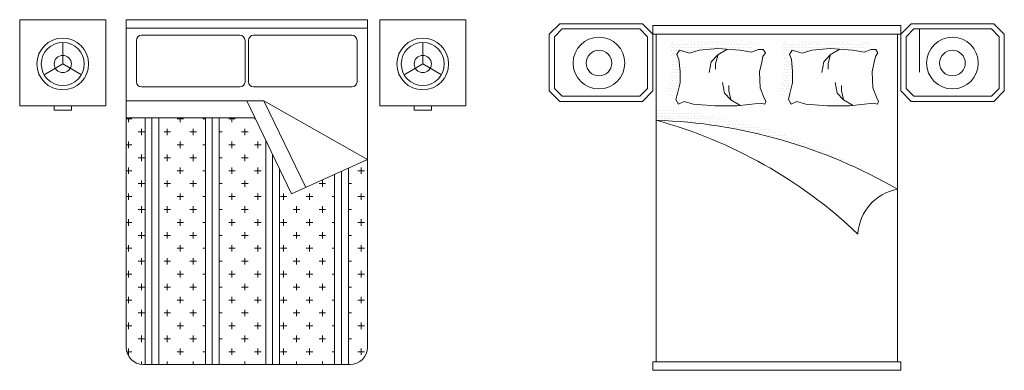
# Model space of a CAD drawing. Units: inches. Extents: x 1994 to 3075, y 3517 to 3950.
# Tile 6 of 58: x 1993.9837 to 1994.2086, y 3553.5954 to 3553.6754. Entities that reach past the tile are written whole.
import ezdxf

# ---------------------------------------------------------------- set-up
doc = ezdxf.new("R2010")
doc.units = ezdxf.units.IN
doc.layers.add('A-FURN-REFR', color=8, linetype='Continuous', lineweight=13)
doc.layers.add('A-FURN-REFR-PATT', color=8, linetype='Continuous', lineweight=13)
pattern_1 = [(360, (1986.051224104058, 3548.643407769799), (0.0003125, 0.000625), [0, -0.000625])]

msp = doc.modelspace()

# ---------------------------------------------------------------- hatches: boundary and pattern name
at = {"layer": 'A-FURN-REFR-PATT'}
h = msp.add_hatch(dxfattribs=at)
h.set_pattern_fill('DOTS', color=256, scale=0.0003937007874016, angle=-1.27e-14, style=0)
h.set_pattern_definition(pattern_1)
h.paths.add_polyline_path([(1994.152040282244, 3553.669850165295), (1994.151555843356, 3553.670576204597), (1994.150465850669, 3553.670576204597), (1994.148891419094, 3553.669971170727), (1994.146227000022, 3553.67045519581), (1994.141140376132, 3553.670818215461), (1994.136901525485, 3553.67045519581), (1994.13472154011, 3553.669729156508), (1994.132420450204, 3553.67045519581), (1994.131814901594, 3553.669487145644), (1994.132299340482, 3553.668398086691), (1994.132541559925, 3553.665614934916), (1994.132541559925, 3553.662952788573), (1994.131936011316, 3553.660532656448), (1994.131572682151, 3553.659201583276), (1994.13217823076, 3553.658112524323), (1994.133510442891, 3553.658717558193), (1994.133909563689, 3553.658600269803), (1994.134507342101, 3553.6609893476), (1994.134507342101, 3553.663651493943), (1994.134265122657, 3553.666434645719), (1994.133780683769, 3553.667523704671), (1994.134386232379, 3553.668491754837), (1994.136687322285, 3553.667765715535), (1994.13886730766, 3553.668491754837), (1994.143106158307, 3553.668854774488), (1994.148192782197, 3553.668491754837), (1994.150857201269, 3553.668007729754), (1994.151283400796, 3553.668171512768), (1994.151434733634, 3553.669003117207)])
h.paths.add_polyline_path([(1994.177760592115, 3553.669850165295), (1994.177276153227, 3553.670576204597), (1994.17618616054, 3553.670576204597), (1994.174611728965, 3553.669971170727), (1994.171947309893, 3553.67045519581), (1994.166860686003, 3553.670818215461), (1994.162621835356, 3553.67045519581), (1994.160441849981, 3553.669729156508), (1994.158140760075, 3553.67045519581), (1994.157535211465, 3553.669487145644), (1994.158019650353, 3553.668398086691), (1994.158261869797, 3553.665614934916), (1994.158261869797, 3553.662952788573), (1994.157656321187, 3553.660532656448), (1994.157292992022, 3553.659201583276), (1994.157898540631, 3553.658112524323), (1994.159230752762, 3553.658717558193), (1994.159629873561, 3553.658600269803), (1994.160227651972, 3553.6609893476), (1994.160227651972, 3553.663651493943), (1994.159985432528, 3553.666434645719), (1994.159500993641, 3553.667523704671), (1994.16010654225, 3553.668491754837), (1994.162407632156, 3553.667765715535), (1994.164587617532, 3553.668491754837), (1994.168826468178, 3553.668854774488), (1994.173913092069, 3553.668491754837), (1994.17657751114, 3553.668007729754), (1994.177003710667, 3553.668171512768), (1994.177155043505, 3553.669003117207)])
h = msp.add_hatch(dxfattribs=at)
h.set_pattern_fill('DOTS', color=256, scale=0.0003937007874016, angle=-1.27e-14, style=0)
h.set_pattern_definition(pattern_1)
h.paths.add_polyline_path([(1994.129055189487, 3553.655169821634), (1994.129055189487, 3553.652470090133, -0.1242730550582239), (1994.184173299723, 3553.636722058637, 0.1225632895340951)])

# ---------------------------------------------------------------- linework, layer by layer
at = {"layer": 'A-FURN-REFR'}
for p, q in [((1993.983652184335, 3553.675442817969), (1994.003337223705, 3553.675442817969)), ((1993.983652184335, 3553.655757778598), (1993.983652184335, 3553.675442817969)), ((1994.003337223705, 3553.675442817969), (1994.003337223705, 3553.655757778598)), ((1994.063084720814, 3553.675442817969), (1994.007966610578, 3553.675442817969)), ((1994.007966610578, 3553.675442817969), (1994.007966610578, 3553.600639668363)), ((1994.063084720814, 3553.600639668363), (1994.063084720814, 3553.675442817969)), ((1994.065893488544, 3553.675442817969), (1994.085578527914, 3553.675442817969)), ((1994.065893488544, 3553.655757778598), (1994.065893488544, 3553.675442817969)), ((1994.085578527914, 3553.675442817969), (1994.085578527914, 3553.655757778598)), ((1994.184960701298, 3553.674123633441), (1994.128267787912, 3553.674123633441)), ((1994.128267787912, 3553.672155129504), (1994.128267787912, 3553.674123633441)), ((1994.184960701298, 3553.674123633441), (1994.184960701298, 3553.672155129504)), ((1994.063084720814, 3553.673474314031), (1994.007966610578, 3553.673474314031)), ((1994.011509917665, 3553.671899510882), (1994.033950862547, 3553.671899510882)), ((1994.059541413728, 3553.671899510882), (1994.037100468846, 3553.671899510882)), ((1994.184960701298, 3553.672155129504), (1994.128267787912, 3553.672155129504)), ((1994.129055189487, 3553.597351979898), (1994.129055189487, 3553.672155129504)), ((1994.184173299723, 3553.672155129504), (1994.184173299723, 3553.597351979898)), ((1994.18919615252, 3553.673293577591), (1994.18919615252, 3553.663451057906)), ((1993.99349470402, 3553.670258471752), (1993.99349470402, 3553.665337211909)), ((1994.010328815302, 3553.661269589622), (1994.010328815302, 3553.670718408521)), ((1994.035131964909, 3553.670718408521), (1994.035131964909, 3553.661269589622)), ((1994.035919366483, 3553.670718408521), (1994.035919366483, 3553.661269589622)), ((1994.06072251609, 3553.661269589622), (1994.06072251609, 3553.670718408521)), ((1994.075736008229, 3553.670258471752), (1994.075736008229, 3553.665337211909)), ((1993.989232767978, 3553.662876581988), (1993.99349470402, 3553.665337211909)), ((1993.997756640062, 3553.662876581988), (1993.99349470402, 3553.665337211909)), ((1994.071474072186, 3553.662876581988), (1994.075736008229, 3553.665337211909)), ((1994.079997944271, 3553.662876581988), (1994.075736008229, 3553.665337211909)), ((1994.033950862547, 3553.66008848726), (1994.011509917665, 3553.66008848726)), ((1994.037100468846, 3553.66008848726), (1994.059541413728, 3553.66008848726)), ((1994.003337223705, 3553.655757778598), (1993.983652184335, 3553.655757778598)), ((1993.991526200083, 3553.654773526631), (1993.991526200083, 3553.655757778598)), ((1993.995463207957, 3553.654773526631), (1993.995463207957, 3553.655757778598)), ((1994.03946267357, 3553.656938880961), (1994.007966610578, 3553.656938880961)), ((1994.045761886168, 3553.635679038441), (1994.035525665696, 3553.656938880961)), ((1994.048991972739, 3553.637147259609), (1994.03946267357, 3553.656938880961)), ((1994.03946267357, 3553.656938880961), (1994.063084720814, 3553.643553054189)), ((1994.085578527914, 3553.655757778598), (1994.065893488544, 3553.655757778598)), ((1994.073767504292, 3553.654773526631), (1994.073767504292, 3553.655757778598)), ((1994.077704512166, 3553.654773526631), (1994.077704512166, 3553.655757778598)), ((1993.995463207957, 3553.654773526631), (1993.991526200083, 3553.654773526631)), ((1994.077704512166, 3553.654773526631), (1994.073767504292, 3553.654773526631)), ((1994.007966610578, 3553.653001873087), (1994.03742126208, 3553.653001873087)), ((1994.009254114629, 3553.652768528092), (1994.007966610578, 3553.652768528092)), ((1994.008515925652, 3553.652030339116), (1994.008515925652, 3553.653001873087)), ((1994.012297319239, 3553.653001873087), (1994.012297319239, 3553.596702660489)), ((1994.013872122389, 3553.653001873087), (1994.013872122389, 3553.596702660489)), ((1994.015446925538, 3553.653001873087), (1994.015446925538, 3553.596702660489)), ((1994.021065138251, 3553.652768528092), (1994.019588760298, 3553.652768528092)), ((1994.020326949274, 3553.652030339116), (1994.020326949274, 3553.653001873087)), ((1994.026076846799, 3553.652768528092), (1994.025494272109, 3553.652768528092)), ((1994.026076846799, 3553.653001873087), (1994.026076846799, 3553.596702660489)), ((1994.027651649948, 3553.653001873087), (1994.027651649948, 3553.596702660489)), ((1994.029226453098, 3553.653001873087), (1994.029226453098, 3553.596702660489)), ((1994.032876161872, 3553.652768528092), (1994.03139978392, 3553.652768528092)), ((1994.032137972896, 3553.652030339116), (1994.032137972896, 3553.653001873087)), ((1994.037533613374, 3553.652768528092), (1994.037305295731, 3553.652768528092)), ((1994.012206870534, 3553.649815772187), (1994.010730492581, 3553.649815772187)), ((1994.011468681558, 3553.64907758321), (1994.011468681558, 3553.650553961162)), ((1994.018112382345, 3553.649815772187), (1994.016636004392, 3553.649815772187)), ((1994.017374193369, 3553.64907758321), (1994.017374193369, 3553.650553961162)), ((1994.024017894156, 3553.649815772187), (1994.022541516203, 3553.649815772187)), ((1994.02327970518, 3553.64907758321), (1994.02327970518, 3553.650553961162)), ((1994.029923405967, 3553.649815772187), (1994.029226453098, 3553.649815772187)), ((1994.035828917778, 3553.649815772187), (1994.034352539825, 3553.649815772187)), ((1994.035090728802, 3553.64907758321), (1994.035090728802, 3553.650553961162)), ((1994.009254114629, 3553.646863016281), (1994.007966610578, 3553.646863016281)), ((1994.008515925652, 3553.646124827305), (1994.008515925652, 3553.647601205258)), ((1994.021065138251, 3553.646863016281), (1994.019588760298, 3553.646863016281)), ((1994.020326949274, 3553.646124827305), (1994.020326949274, 3553.647601205258)), ((1994.026076846799, 3553.646863016281), (1994.025494272109, 3553.646863016281)), ((1994.032876161872, 3553.646863016281), (1994.03139978392, 3553.646863016281)), ((1994.032137972896, 3553.646124827305), (1994.032137972896, 3553.647601205258)), ((1994.038781673683, 3553.646863016281), (1994.037305295731, 3553.646863016281)), ((1994.038043484707, 3553.646124827305), (1994.038043484707, 3553.647601205258)), ((1994.039856374358, 3553.647944332202), (1994.039856374358, 3553.596702660489)), ((1994.011468681558, 3553.643172071399), (1994.011468681558, 3553.644648449352)), ((1994.017374193369, 3553.643172071399), (1994.017374193369, 3553.644648449352)), ((1994.02327970518, 3553.643172071399), (1994.02327970518, 3553.644648449352)), ((1994.035090728802, 3553.643172071399), (1994.035090728802, 3553.644648449352)), ((1994.041431177507, 3553.6446735872), (1994.041431177507, 3553.596702660489)), ((1994.012206870534, 3553.643910260375), (1994.010730492581, 3553.643910260375)), ((1994.018112382345, 3553.643910260375), (1994.016636004392, 3553.643910260375)), ((1994.024017894156, 3553.643910260375), (1994.022541516203, 3553.643910260375)), ((1994.029923405967, 3553.643910260375), (1994.029226453098, 3553.643910260375)), ((1994.035828917778, 3553.643910260375), (1994.034352539825, 3553.643910260375)), ((1994.063084720814, 3553.643553054189), (1994.045761886168, 3553.635679038441)), ((1994.009254114629, 3553.64095750447), (1994.007966610578, 3553.64095750447)), ((1994.008515925652, 3553.640219315493), (1994.008515925652, 3553.641695693446)), ((1994.021065138251, 3553.64095750447), (1994.019588760298, 3553.64095750447)), ((1994.020326949274, 3553.640219315493), (1994.020326949274, 3553.641695693446)), ((1994.026076846799, 3553.64095750447), (1994.025494272109, 3553.64095750447)), ((1994.032876161872, 3553.64095750447), (1994.03139978392, 3553.64095750447)), ((1994.032137972896, 3553.640219315493), (1994.032137972896, 3553.641695693446)), ((1994.038781673683, 3553.64095750447), (1994.037305295731, 3553.64095750447)), ((1994.038043484707, 3553.640219315493), (1994.038043484707, 3553.641695693446)), ((1994.043005980657, 3553.641402842197), (1994.043005980657, 3553.596702660489)), ((1994.043220402525, 3553.64095750447), (1994.043210807542, 3553.64095750447)), ((1994.055604405854, 3553.640152911026), (1994.055604405854, 3553.596702660489)), ((1994.057179209003, 3553.640868730639), (1994.057179209003, 3553.596702660489)), ((1994.058754012153, 3553.641584550252), (1994.058754012153, 3553.596702660489)), ((1994.062403720928, 3553.64095750447), (1994.060927342975, 3553.64095750447)), ((1994.061665531951, 3553.640219315493), (1994.061665531951, 3553.641695693446)), ((1994.012206870534, 3553.638004748564), (1994.010730492581, 3553.638004748564)), ((1994.011468681558, 3553.637266559588), (1994.011468681558, 3553.63874293754)), ((1994.018112382345, 3553.638004748564), (1994.016636004392, 3553.638004748564)), ((1994.017374193369, 3553.637266559588), (1994.017374193369, 3553.63874293754)), ((1994.024017894156, 3553.638004748564), (1994.022541516203, 3553.638004748564)), ((1994.02327970518, 3553.637266559588), (1994.02327970518, 3553.63874293754)), ((1994.029923405967, 3553.638004748564), (1994.029226453098, 3553.638004748564)), ((1994.035828917778, 3553.638004748564), (1994.034352539825, 3553.638004748564)), ((1994.035090728802, 3553.637266559588), (1994.035090728802, 3553.63874293754)), ((1994.053545453211, 3553.638004748564), (1994.052069075259, 3553.638004748564)), ((1994.052807264235, 3553.637266559588), (1994.052807264235, 3553.63874293754)), ((1994.059450965022, 3553.638004748564), (1994.058754012153, 3553.638004748564)), ((1994.008515925652, 3553.634313803683), (1994.008515925652, 3553.635790181636)), ((1994.020326949274, 3553.634313803683), (1994.020326949274, 3553.635790181636)), ((1994.032137972896, 3553.634313803683), (1994.032137972896, 3553.635790181636)), ((1994.038043484707, 3553.634313803683), (1994.038043484707, 3553.635790181636)), ((1994.043948996518, 3553.634313803683), (1994.043948996518, 3553.635790181636)), ((1994.049854508329, 3553.634313803683), (1994.049854508329, 3553.635790181636)), ((1994.061665531951, 3553.634313803683), (1994.061665531951, 3553.635790181636)), ((1994.009254114629, 3553.635051992659), (1994.007966610578, 3553.635051992659)), ((1994.021065138251, 3553.635051992659), (1994.019588760298, 3553.635051992659)), ((1994.026076846799, 3553.635051992659), (1994.025494272109, 3553.635051992659)), ((1994.032876161872, 3553.635051992659), (1994.03139978392, 3553.635051992659)), ((1994.038781673683, 3553.635051992659), (1994.037305295731, 3553.635051992659)), ((1994.044687185495, 3553.635051992659), (1994.043210807542, 3553.635051992659)), ((1994.050592697306, 3553.635051992659), (1994.049116319353, 3553.635051992659)), ((1994.055604405854, 3553.635051992659), (1994.055021831164, 3553.635051992659)), ((1994.062403720928, 3553.635051992659), (1994.060927342975, 3553.635051992659)), ((1994.012206870534, 3553.632099236754), (1994.010730492581, 3553.632099236754)), ((1994.011468681558, 3553.631361047777), (1994.011468681558, 3553.632837425729)), ((1994.018112382345, 3553.632099236754), (1994.016636004392, 3553.632099236754)), ((1994.017374193369, 3553.631361047777), (1994.017374193369, 3553.632837425729)), ((1994.024017894156, 3553.632099236754), (1994.022541516203, 3553.632099236754)), ((1994.02327970518, 3553.631361047777), (1994.02327970518, 3553.632837425729)), ((1994.029923405967, 3553.632099236754), (1994.029226453098, 3553.632099236754)), ((1994.035828917778, 3553.632099236754), (1994.034352539825, 3553.632099236754)), ((1994.035090728802, 3553.631361047777), (1994.035090728802, 3553.632837425729)), ((1994.0476399414, 3553.632099236754), (1994.046163563448, 3553.632099236754)), ((1994.046901752424, 3553.631361047777), (1994.046901752424, 3553.632837425729)), ((1994.053545453211, 3553.632099236754), (1994.052069075259, 3553.632099236754)), ((1994.052807264235, 3553.631361047777), (1994.052807264235, 3553.632837425729)), ((1994.059450965022, 3553.632099236754), (1994.058754012153, 3553.632099236754)), ((1994.009254114629, 3553.629146480847), (1994.007966610578, 3553.629146480847)), ((1994.008515925652, 3553.628408291871), (1994.008515925652, 3553.629884669824)), ((1994.021065138251, 3553.629146480847), (1994.019588760298, 3553.629146480847)), ((1994.020326949274, 3553.628408291871), (1994.020326949274, 3553.629884669824)), ((1994.026076846799, 3553.629146480847), (1994.025494272109, 3553.629146480847)), ((1994.032876161872, 3553.629146480847), (1994.03139978392, 3553.629146480847)), ((1994.032137972896, 3553.628408291871), (1994.032137972896, 3553.629884669824)), ((1994.038781673683, 3553.629146480847), (1994.037305295731, 3553.629146480847)), ((1994.038043484707, 3553.628408291871), (1994.038043484707, 3553.629884669824)), ((1994.044687185495, 3553.629146480847), (1994.043210807542, 3553.629146480847)), ((1994.043948996518, 3553.628408291871), (1994.043948996518, 3553.629884669824)), ((1994.050592697306, 3553.629146480847), (1994.049116319353, 3553.629146480847)), ((1994.049854508329, 3553.628408291871), (1994.049854508329, 3553.629884669824)), ((1994.055604405854, 3553.629146480847), (1994.055021831164, 3553.629146480847)), ((1994.062403720928, 3553.629146480847), (1994.060927342975, 3553.629146480847)), ((1994.061665531951, 3553.628408291871), (1994.061665531951, 3553.629884669824)), ((1994.011468681558, 3553.625455535966), (1994.011468681558, 3553.626931913919)), ((1994.017374193369, 3553.625455535966), (1994.017374193369, 3553.626931913919)), ((1994.02327970518, 3553.625455535966), (1994.02327970518, 3553.626931913919)), ((1994.035090728802, 3553.625455535966), (1994.035090728802, 3553.626931913919)), ((1994.046901752424, 3553.625455535966), (1994.046901752424, 3553.626931913919)), ((1994.052807264235, 3553.625455535966), (1994.052807264235, 3553.626931913919)), ((1994.012206870534, 3553.626193724942), (1994.010730492581, 3553.626193724942)), ((1994.018112382345, 3553.626193724942), (1994.016636004392, 3553.626193724942)), ((1994.024017894156, 3553.626193724942), (1994.022541516203, 3553.626193724942)), ((1994.029923405967, 3553.626193724942), (1994.029226453098, 3553.626193724942)), ((1994.035828917778, 3553.626193724942), (1994.034352539825, 3553.626193724942)), ((1994.0476399414, 3553.626193724942), (1994.046163563448, 3553.626193724942)), ((1994.053545453211, 3553.626193724942), (1994.052069075259, 3553.626193724942)), ((1994.059450965022, 3553.626193724942), (1994.058754012153, 3553.626193724942)), ((1994.009254114629, 3553.623240969037), (1994.007966610578, 3553.623240969037)), ((1994.008515925652, 3553.62250278006), (1994.008515925652, 3553.623979158013)), ((1994.021065138251, 3553.623240969037), (1994.019588760298, 3553.623240969037)), ((1994.020326949274, 3553.62250278006), (1994.020326949274, 3553.623979158013)), ((1994.026076846799, 3553.623240969037), (1994.025494272109, 3553.623240969037)), ((1994.032876161872, 3553.623240969037), (1994.03139978392, 3553.623240969037)), ((1994.032137972896, 3553.62250278006), (1994.032137972896, 3553.623979158013)), ((1994.038781673683, 3553.623240969037), (1994.037305295731, 3553.623240969037)), ((1994.038043484707, 3553.62250278006), (1994.038043484707, 3553.623979158013)), ((1994.044687185495, 3553.623240969037), (1994.043210807542, 3553.623240969037)), ((1994.043948996518, 3553.62250278006), (1994.043948996518, 3553.623979158013)), ((1994.050592697306, 3553.623240969037), (1994.049116319353, 3553.623240969037)), ((1994.049854508329, 3553.62250278006), (1994.049854508329, 3553.623979158013)), ((1994.055604405854, 3553.623240969037), (1994.055021831164, 3553.623240969037)), ((1994.062403720928, 3553.623240969037), (1994.060927342975, 3553.623240969037)), ((1994.061665531951, 3553.62250278006), (1994.061665531951, 3553.623979158013)), ((1994.012206870534, 3553.620288213132), (1994.010730492581, 3553.620288213132)), ((1994.011468681558, 3553.619550024155), (1994.011468681558, 3553.621026402107)), ((1994.018112382345, 3553.620288213132), (1994.016636004392, 3553.620288213132)), ((1994.017374193369, 3553.619550024155), (1994.017374193369, 3553.621026402107)), ((1994.024017894156, 3553.620288213132), (1994.022541516203, 3553.620288213132)), ((1994.02327970518, 3553.619550024155), (1994.02327970518, 3553.621026402107)), ((1994.029923405967, 3553.620288213132), (1994.029226453098, 3553.620288213132)), ((1994.035828917778, 3553.620288213132), (1994.034352539825, 3553.620288213132)), ((1994.035090728802, 3553.619550024155), (1994.035090728802, 3553.621026402107)), ((1994.0476399414, 3553.620288213132), (1994.046163563448, 3553.620288213132)), ((1994.046901752424, 3553.619550024155), (1994.046901752424, 3553.621026402107)), ((1994.053545453211, 3553.620288213132), (1994.052069075259, 3553.620288213132)), ((1994.052807264235, 3553.619550024155), (1994.052807264235, 3553.621026402107)), ((1994.059450965022, 3553.620288213132), (1994.058754012153, 3553.620288213132)), ((1994.009254114629, 3553.617335457226), (1994.007966610578, 3553.617335457226)), ((1994.008515925652, 3553.61659726825), (1994.008515925652, 3553.618073646202)), ((1994.021065138251, 3553.617335457226), (1994.019588760298, 3553.617335457226)), ((1994.020326949274, 3553.61659726825), (1994.020326949274, 3553.618073646202)), ((1994.026076846799, 3553.617335457226), (1994.025494272109, 3553.617335457226)), ((1994.032876161872, 3553.617335457226), (1994.03139978392, 3553.617335457226)), ((1994.032137972896, 3553.61659726825), (1994.032137972896, 3553.618073646202)), ((1994.038781673683, 3553.617335457226), (1994.037305295731, 3553.617335457226)), ((1994.038043484707, 3553.61659726825), (1994.038043484707, 3553.618073646202)), ((1994.044687185495, 3553.617335457226), (1994.043210807542, 3553.617335457226)), ((1994.043948996518, 3553.61659726825), (1994.043948996518, 3553.618073646202)), ((1994.050592697306, 3553.617335457226), (1994.049116319353, 3553.617335457226)), ((1994.049854508329, 3553.61659726825), (1994.049854508329, 3553.618073646202)), ((1994.055604405854, 3553.617335457226), (1994.055021831164, 3553.617335457226)), ((1994.062403720928, 3553.617335457226), (1994.060927342975, 3553.617335457226)), ((1994.061665531951, 3553.61659726825), (1994.061665531951, 3553.618073646202)), ((1994.011468681558, 3553.613644512343), (1994.011468681558, 3553.615120890297)), ((1994.017374193369, 3553.613644512343), (1994.017374193369, 3553.615120890297)), ((1994.02327970518, 3553.613644512343), (1994.02327970518, 3553.615120890297)), ((1994.035090728802, 3553.613644512343), (1994.035090728802, 3553.615120890297)), ((1994.046901752424, 3553.613644512343), (1994.046901752424, 3553.615120890297)), ((1994.052807264235, 3553.613644512343), (1994.052807264235, 3553.615120890297)), ((1994.012206870534, 3553.61438270132), (1994.010730492581, 3553.61438270132)), ((1994.018112382345, 3553.61438270132), (1994.016636004392, 3553.61438270132)), ((1994.024017894156, 3553.61438270132), (1994.022541516203, 3553.61438270132)), ((1994.029923405967, 3553.61438270132), (1994.029226453098, 3553.61438270132)), ((1994.035828917778, 3553.61438270132), (1994.034352539825, 3553.61438270132)), ((1994.0476399414, 3553.61438270132), (1994.046163563448, 3553.61438270132)), ((1994.053545453211, 3553.61438270132), (1994.052069075259, 3553.61438270132)), ((1994.059450965022, 3553.61438270132), (1994.058754012153, 3553.61438270132)), ((1994.009254114629, 3553.611429945414), (1994.007966610578, 3553.611429945414)), ((1994.008515925652, 3553.610691756438), (1994.008515925652, 3553.612168134391)), ((1994.021065138251, 3553.611429945414), (1994.019588760298, 3553.611429945414)), ((1994.020326949274, 3553.610691756438), (1994.020326949274, 3553.612168134391)), ((1994.026076846799, 3553.611429945414), (1994.025494272109, 3553.611429945414)), ((1994.032876161872, 3553.611429945414), (1994.03139978392, 3553.611429945414)), ((1994.032137972896, 3553.610691756438), (1994.032137972896, 3553.612168134391)), ((1994.038781673683, 3553.611429945414), (1994.037305295731, 3553.611429945414)), ((1994.038043484707, 3553.610691756438), (1994.038043484707, 3553.612168134391)), ((1994.044687185495, 3553.611429945414), (1994.043210807542, 3553.611429945414)), ((1994.043948996518, 3553.610691756438), (1994.043948996518, 3553.612168134391)), ((1994.050592697306, 3553.611429945414), (1994.049116319353, 3553.611429945414)), ((1994.049854508329, 3553.610691756438), (1994.049854508329, 3553.612168134391)), ((1994.055604405854, 3553.611429945414), (1994.055021831164, 3553.611429945414)), ((1994.062403720928, 3553.611429945414), (1994.060927342975, 3553.611429945414)), ((1994.061665531951, 3553.610691756438), (1994.061665531951, 3553.612168134391)), ((1994.012206870534, 3553.608477189509), (1994.010730492581, 3553.608477189509)), ((1994.011468681558, 3553.607739000533), (1994.011468681558, 3553.609215378486)), ((1994.018112382345, 3553.608477189509), (1994.016636004392, 3553.608477189509)), ((1994.017374193369, 3553.607739000533), (1994.017374193369, 3553.609215378486)), ((1994.024017894156, 3553.608477189509), (1994.022541516203, 3553.608477189509)), ((1994.02327970518, 3553.607739000533), (1994.02327970518, 3553.609215378486)), ((1994.029923405967, 3553.608477189509), (1994.029226453098, 3553.608477189509)), ((1994.035828917778, 3553.608477189509), (1994.034352539825, 3553.608477189509)), ((1994.035090728802, 3553.607739000533), (1994.035090728802, 3553.609215378486)), ((1994.0476399414, 3553.608477189509), (1994.046163563448, 3553.608477189509)), ((1994.046901752424, 3553.607739000533), (1994.046901752424, 3553.609215378486)), ((1994.053545453211, 3553.608477189509), (1994.052069075259, 3553.608477189509)), ((1994.052807264235, 3553.607739000533), (1994.052807264235, 3553.609215378486)), ((1994.059450965022, 3553.608477189509), (1994.058754012153, 3553.608477189509)), ((1994.008515925652, 3553.604786244628), (1994.008515925652, 3553.60626262258)), ((1994.020326949274, 3553.604786244628), (1994.020326949274, 3553.60626262258)), ((1994.032137972896, 3553.604786244628), (1994.032137972896, 3553.60626262258)), ((1994.038043484707, 3553.604786244628), (1994.038043484707, 3553.60626262258)), ((1994.043948996518, 3553.604786244628), (1994.043948996518, 3553.60626262258)), ((1994.049854508329, 3553.604786244628), (1994.049854508329, 3553.60626262258)), ((1994.061665531951, 3553.604786244628), (1994.061665531951, 3553.60626262258)), ((1994.009254114629, 3553.605524433603), (1994.007966610578, 3553.605524433603)), ((1994.021065138251, 3553.605524433603), (1994.019588760298, 3553.605524433603)), ((1994.026076846799, 3553.605524433603), (1994.025494272109, 3553.605524433603)), ((1994.032876161872, 3553.605524433603), (1994.03139978392, 3553.605524433603)), ((1994.038781673683, 3553.605524433603), (1994.037305295731, 3553.605524433603)), ((1994.044687185495, 3553.605524433603), (1994.043210807542, 3553.605524433603)), ((1994.050592697306, 3553.605524433603), (1994.049116319353, 3553.605524433603)), ((1994.055604405854, 3553.605524433603), (1994.055021831164, 3553.605524433603)), ((1994.062403720928, 3553.605524433603), (1994.060927342975, 3553.605524433603)), ((1994.012206870534, 3553.602571677699), (1994.010730492581, 3553.602571677699)), ((1994.011468681558, 3553.601833488722), (1994.011468681558, 3553.603309866674)), ((1994.018112382345, 3553.602571677699), (1994.016636004392, 3553.602571677699)), ((1994.017374193369, 3553.601833488722), (1994.017374193369, 3553.603309866674)), ((1994.024017894156, 3553.602571677699), (1994.022541516203, 3553.602571677699)), ((1994.02327970518, 3553.601833488722), (1994.02327970518, 3553.603309866674)), ((1994.029923405967, 3553.602571677699), (1994.029226453098, 3553.602571677699)), ((1994.035828917778, 3553.602571677699), (1994.034352539825, 3553.602571677699)), ((1994.035090728802, 3553.601833488722), (1994.035090728802, 3553.603309866674)), ((1994.0476399414, 3553.602571677699), (1994.046163563448, 3553.602571677699)), ((1994.046901752424, 3553.601833488722), (1994.046901752424, 3553.603309866674)), ((1994.053545453211, 3553.602571677699), (1994.052069075259, 3553.602571677699)), ((1994.052807264235, 3553.601833488722), (1994.052807264235, 3553.603309866674)), ((1994.059450965022, 3553.602571677699), (1994.058754012153, 3553.602571677699)), ((1994.009254114629, 3553.599618921793), (1994.00810123664, 3553.599618921793)), ((1994.008515925652, 3553.598880732816), (1994.008515925652, 3553.600357110769)), ((1994.021065138251, 3553.599618921793), (1994.019588760298, 3553.599618921793)), ((1994.020326949274, 3553.598880732816), (1994.020326949274, 3553.600357110769)), ((1994.026076846799, 3553.599618921793), (1994.025494272109, 3553.599618921793)), ((1994.032876161872, 3553.599618921793), (1994.03139978392, 3553.599618921793)), ((1994.032137972896, 3553.598880732816), (1994.032137972896, 3553.600357110769)), ((1994.038781673683, 3553.599618921793), (1994.037305295731, 3553.599618921793)), ((1994.038043484707, 3553.598880732816), (1994.038043484707, 3553.600357110769)), ((1994.044687185495, 3553.599618921793), (1994.043210807542, 3553.599618921793)), ((1994.043948996518, 3553.598880732816), (1994.043948996518, 3553.600357110769)), ((1994.050592697306, 3553.599618921793), (1994.049116319353, 3553.599618921793)), ((1994.049854508329, 3553.598880732816), (1994.049854508329, 3553.600357110769)), ((1994.055604405854, 3553.599618921793), (1994.055021831164, 3553.599618921793)), ((1994.062403720928, 3553.599618921793), (1994.060927342975, 3553.599618921793)), ((1994.061665531951, 3553.598880732816), (1994.061665531951, 3553.600357110769)), ((1994.011468681558, 3553.596726758844), (1994.011468681558, 3553.597404354864)), ((1994.017374193369, 3553.596702660489), (1994.017374193369, 3553.597404354864)), ((1994.02327970518, 3553.596702660489), (1994.02327970518, 3553.597404354864)), ((1994.035090728802, 3553.596702660489), (1994.035090728802, 3553.597404354864)), ((1994.046901752424, 3553.596702660489), (1994.046901752424, 3553.597404354864)), ((1994.052807264235, 3553.596702660489), (1994.052807264235, 3553.597404354864)), ((1994.184960701298, 3553.597351979898), (1994.128267787912, 3553.597351979898)), ((1994.128267787912, 3553.59538347596), (1994.128267787912, 3553.597351979898)), ((1994.184960701298, 3553.597351979898), (1994.184960701298, 3553.59538347596)), ((1994.011903618452, 3553.596702660489), (1994.05914771294, 3553.596702660489)), ((1994.184960701298, 3553.59538347596), (1994.128267787912, 3553.59538347596))]:
    msp.add_line(p, q, dxfattribs=at)
for points in [[(1994.107007945393, 3553.656800798795), (1994.125905583188, 3553.656800798795), (1994.128267787912, 3553.659163003519), (1994.128267787912, 3553.672155129504), (1994.125905583188, 3553.674517334228), (1994.107007945393, 3553.674517334228), (1994.104645740668, 3553.672155129504), (1994.104645740668, 3553.659163003519)], [(1994.187322906023, 3553.656800798795), (1994.206220543818, 3553.656800798795), (1994.208582748542, 3553.659163003519), (1994.208582748542, 3553.672155129504), (1994.206220543818, 3553.674517334228), (1994.187322906023, 3553.674517334228), (1994.184960701298, 3553.672155129504), (1994.184960701298, 3553.659163003519)], [(1994.107598496574, 3553.657981901157), (1994.125315032007, 3553.657981901157), (1994.12708668555, 3553.6597535547), (1994.12708668555, 3553.671564578323), (1994.125315032007, 3553.673336231866), (1994.107598496574, 3553.673336231866), (1994.10582684303, 3553.671564578323), (1994.10582684303, 3553.6597535547)], [(1994.187913457204, 3553.657981901157), (1994.205629992636, 3553.657981901157), (1994.20740164618, 3553.6597535547), (1994.20740164618, 3553.671564578323), (1994.205629992636, 3553.673336231866), (1994.187913457204, 3553.673336231866), (1994.18614180366, 3553.671564578323), (1994.18614180366, 3553.6597535547)]]:
    msp.add_lwpolyline(points, close=True, dxfattribs=at)
for points in [[(1994.136687322285, 3553.667765715535), (1994.134386232379, 3553.668491754837), (1994.133780683769, 3553.667523704671), (1994.134265122657, 3553.666434645719), (1994.134507342101, 3553.663651493943), (1994.134507342101, 3553.6609893476), (1994.133901793492, 3553.658569215475), (1994.133538464326, 3553.657238142303), (1994.134144012935, 3553.656149083351), (1994.135476225067, 3553.65675411722), (1994.137535095529, 3553.656149083351), (1994.142500609697, 3553.6557860637), (1994.147587228397, 3553.6557860637), (1994.152916071731, 3553.65639109757), (1994.153884954697, 3553.656149083351), (1994.154127174141, 3553.65675411722), (1994.153642735254, 3553.657722167386), (1994.15279496201, 3553.659900288647), (1994.152673852288, 3553.663530485156), (1994.153158291175, 3553.665708603062), (1994.15340051581, 3553.667039676233), (1994.154006064419, 3553.667886724323), (1994.153521625532, 3553.668612763624), (1994.152431632844, 3553.668612763624), (1994.150857201269, 3553.668007729754), (1994.148192782197, 3553.668491754837), (1994.143106158307, 3553.668854774488), (1994.13886730766, 3553.668491754837), (1994.136687322285, 3553.667765715535)], [(1994.145165028769, 3553.668612763624), (1994.143106158307, 3553.667402695884), (1994.141652836454, 3553.665829611849), (1994.141168397566, 3553.663409479725)], [(1994.143106158307, 3553.667281690453), (1994.142621719419, 3553.665345583411), (1994.142621719419, 3553.664135519027)], [(1994.162407632156, 3553.667765715535), (1994.16010654225, 3553.668491754837), (1994.159500993641, 3553.667523704671), (1994.159985432528, 3553.666434645719), (1994.160227651972, 3553.663651493943), (1994.160227651972, 3553.6609893476), (1994.159622103363, 3553.658569215475), (1994.159258774197, 3553.657238142303), (1994.159864322807, 3553.656149083351), (1994.161196534938, 3553.65675411722), (1994.1632554054, 3553.656149083351), (1994.168220919569, 3553.6557860637), (1994.173307538268, 3553.6557860637), (1994.178636381603, 3553.65639109757), (1994.179605264568, 3553.656149083351), (1994.179847484012, 3553.65675411722), (1994.179363045125, 3553.657722167386), (1994.178515271881, 3553.659900288647), (1994.178394162159, 3553.663530485156), (1994.178878601046, 3553.665708603062), (1994.179120825681, 3553.667039676233), (1994.17972637429, 3553.667886724323), (1994.179241935403, 3553.668612763624), (1994.178151942715, 3553.668612763624), (1994.17657751114, 3553.668007729754), (1994.173913092069, 3553.668491754837), (1994.168826468178, 3553.668854774488), (1994.164587617532, 3553.668491754837), (1994.162407632156, 3553.667765715535)], [(1994.17088533864, 3553.668612763624), (1994.168826468178, 3553.667402695884), (1994.167373146325, 3553.665829611849), (1994.166888707438, 3553.663409479725)], [(1994.168826468178, 3553.667281690453), (1994.168342029291, 3553.665345583411), (1994.168342029291, 3553.664135519027)], [(1994.148192777007, 3553.655907069132), (1994.146133906544, 3553.657117136872), (1994.144680584691, 3553.658690220907), (1994.144196145804, 3553.661110353032)], [(1994.146133906544, 3553.657238142303), (1994.145649467657, 3553.659174249345), (1994.145649467657, 3553.660384313729)], [(1994.173913086878, 3553.655907069132), (1994.171854216415, 3553.657117136872), (1994.170400894562, 3553.658690220907), (1994.169916455675, 3553.661110353032)], [(1994.171854216415, 3553.657238142303), (1994.171369777528, 3553.659174249345), (1994.171369777528, 3553.660384313729)]]:
    msp.add_lwpolyline(points, dxfattribs=at)
for centre, radius in [((1993.99349470402, 3553.665337211909), 0.0059055118110236), ((1994.075736008229, 3553.665337211909), 0.0059055118110236), ((1994.115984665347, 3553.665539113755), 0.0059055118110236), ((1994.19674002273, 3553.665539113755), 0.0059055118110236), ((1993.99349470402, 3553.665337211909), 0.0049212598425197), ((1994.075736008229, 3553.665337211909), 0.0049212598425197), ((1993.99349470402, 3553.665337211909), 0.0019685039370079), ((1994.075736008229, 3553.665337211909), 0.0019685039370079), ((1994.115984665347, 3553.665539113755), 0.002925824490266), ((1994.19674002273, 3553.665539113755), 0.002925824490266)]:
    msp.add_circle(centre, radius, dxfattribs=at)
for centre, radius, start, end in [((1994.011509917665, 3553.670718408521), 0.0011811023622047, 90, 180), ((1994.033950862547, 3553.670718408521), 0.0011811023622047, 0, 90), ((1994.037100468846, 3553.670718408521), 0.0011811023622047, 90, 180), ((1994.059541413728, 3553.670718408521), 0.0011811023622047, 0, 90), ((1994.011509917665, 3553.661269589622), 0.0011811023622047, 180, 270), ((1994.033950862547, 3553.661269589622), 0.0011811023622047, 270, 0), ((1994.037100468846, 3553.661269589622), 0.0011811023622047, 180, 270), ((1994.059541413728, 3553.661269589622), 0.0011811023622047, 270, 0), ((1994.125423206929, 3553.535427442519), 0.1170989865798539, 59.88659891512252, 88.22260928316399), ((1994.10053202563, 3553.548039700916), 0.1082556098713949, 46.4366712848061, 74.72335959774351), ((1994.186157116233, 3553.625864346196), 0.0110374565646605, 100.3543207538396, 176.786172072198), ((1994.011903618452, 3553.600639668363), 0.0039370078740157, 180, 270), ((1994.05914771294, 3553.600639668363), 0.0039370078740157, 270, 0)]:
    msp.add_arc(centre, radius, start, end, dxfattribs=at)

doc.saveas('drawing.dxf')
